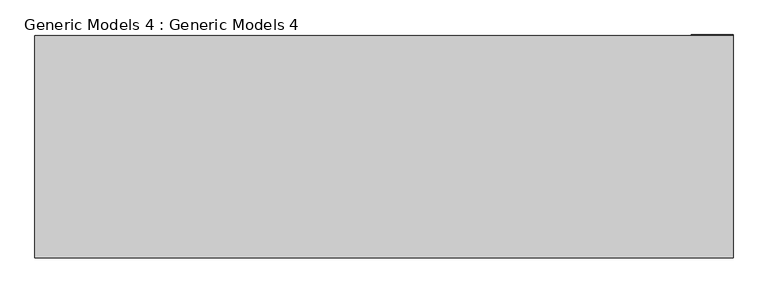
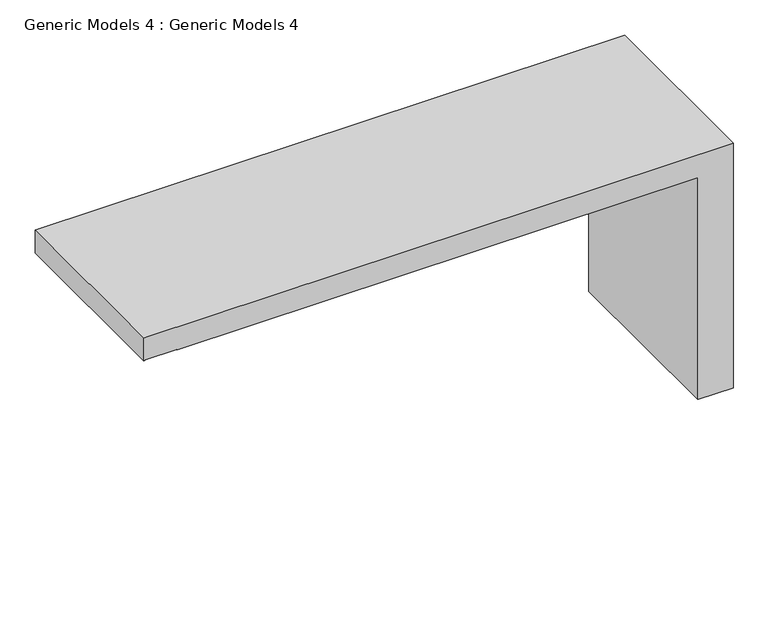
"""IFC4 building model written with IfcOpenShell, lengths in millimetres: proxy geometry, Generic Models 4 : Generic Models 4."""

from ifc_helpers import new_model, si_unit, origin, place, context, project, spatial, faceted_brep, source, transform, mapped, element, save


def generic_models_4_generic_models_4_e1efe8a4(model_context):
    return source(origin(), model_context, "Body", "Brep", [
        faceted_brep([(-17013.5071742, -13196.1337862, 9765.4359555), (-17013.5071742, -15638.5742702, 9765.4359555), (-9360.4652876, -15638.5742702, 9765.4359555), (-9360.4652876, -13196.1337862, 9765.4359555), (-17013.5071742, -15638.5742702, 9451.4798658), (-17013.5071742, -13196.1337862, 9451.4798658), (-17001.1767684, -13196.1337862, 9451.4798658), (-17001.1767684, -15638.5742702, 9451.4798658), (-9360.4652876, -13196.1337862, 9460.6359555), (-9817.6652876, -13196.1337862, 9460.6359555), (-9817.6652876, -13196.1337862, 9451.4798658), (-16587.1168969, -13196.1337862, 9451.4798658), (-16587.1168969, -13196.1337862, 9460.6359555), (-17001.1767684, -13196.1337862, 9460.6359555), (-9360.4652876, -13188.7837464, 9460.6359555), (-9817.6652876, -13188.7837464, 9460.6359555), (-9360.4652876, -15638.5742702, 6400.8), (-9817.6652876, -15638.5742702, 6400.8), (-9817.6652876, -13188.7837464, 6400.8), (-9360.4652876, -13188.7837464, 6400.8), (-9817.6652876, -15638.5742702, 9451.4798658), (-17001.1767684, -15638.5742702, 9460.6359555), (-16587.1168969, -15638.5742702, 9460.6359555), (-16587.1168969, -15638.5742702, 9451.4798658), (-16587.1168969, -15333.7742702, 9460.6359555), (-17001.1767684, -15333.7742702, 9460.6359555)], [[[0, 1, 2, 3]], [[4, 5, 6, 7]], [[1, 0, 5, 4]], [[0, 3, 8, 9, 10, 11, 12, 13, 6, 5]], [[14, 15, 9, 8]], [[16, 17, 18, 19]], [[3, 2, 16, 19, 14, 8]], [[15, 14, 19, 18]], [[18, 17, 20, 10, 9, 15]], [[2, 1, 4, 7, 21, 22, 23, 20, 17, 16]], [[13, 12, 24, 22, 21, 25]], [[12, 11, 23, 22, 24]], [[6, 13, 25, 21, 7]], [[10, 20, 23, 11]]]),
    ])


if __name__ == "__main__":
    model = new_model("IFC4")
    model_context = context("Model", 3, world=origin())
    ifc_project = project(units=[si_unit("LENGTHUNIT", "METRE", prefix="MILLI")], contexts=[model_context])
    site = spatial("IfcSite", under=ifc_project)
    building = spatial("IfcBuilding", under=site)
    placement = place(None, origin())
    generic_models_4_generic_models_4_shape = generic_models_4_generic_models_4_e1efe8a4(model_context)
    element("IfcBuildingElementProxy", 1, Name="Generic Models 4 : Generic Models 4", ObjectType="Generic Models 4 : Generic Models 4", at=placement, inside=building, context=model_context, shape_type="MappedRepresentation", body=[
        mapped(generic_models_4_generic_models_4_shape, transform((0.0, 0.0, 0.0), x_axis=(1.0, 0.0, 0.0), y_axis=(0.0, 1.0, 0.0), z_axis=(0.0, 0.0, 1.0))),
    ])
    save(model, "model.ifc")
